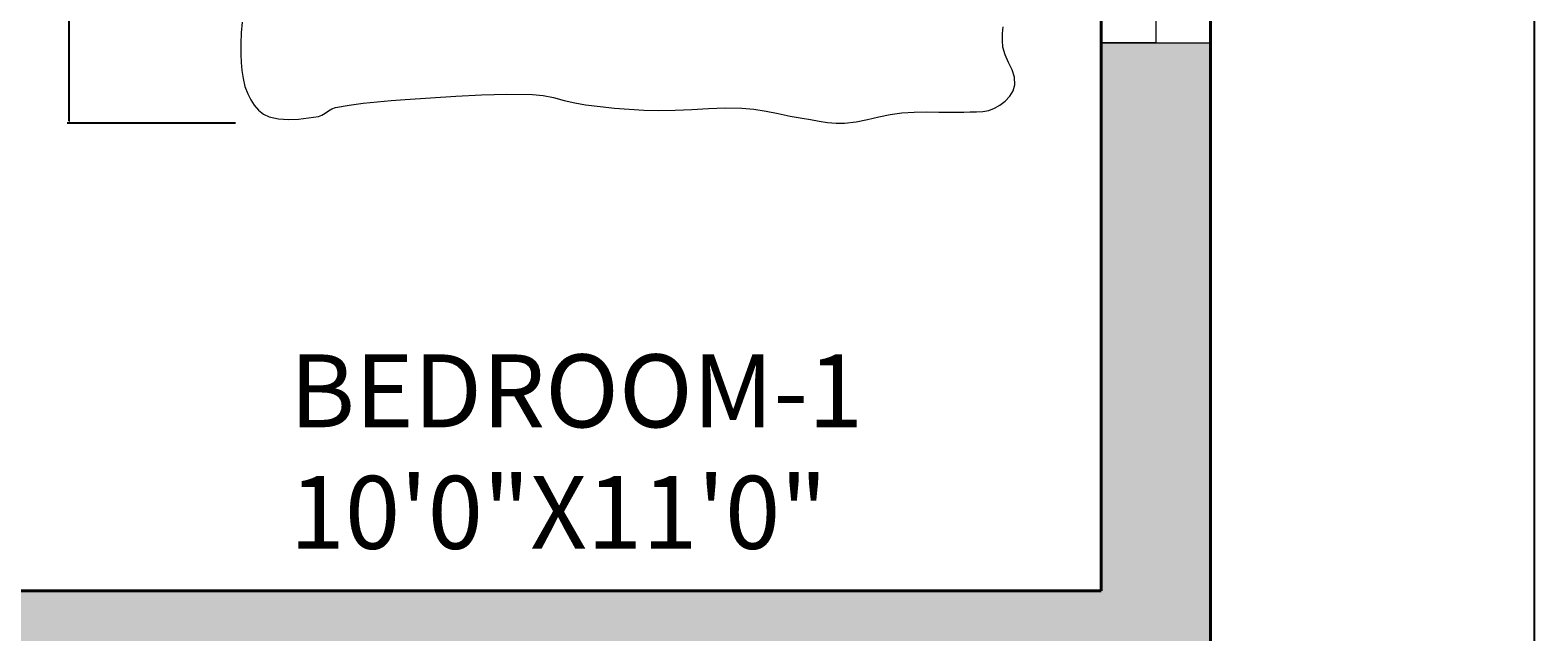
# Model space of a CAD drawing. Units: inches. Extents: x 1441 to 2460, y 1648 to 2683.
# Tile 22 of 35: x 1792 to 1916, y 2154 to 2204. Entities that reach past the tile are written whole.
import ezdxf

# ---------------------------------------------------------------- set-up
doc = ezdxf.new("R2010")
doc.units = ezdxf.units.IN
for name, color, linetype, lineweight in [('A-ANNO-DIMS', 2, 'Continuous', 18), ('A-AREA-IDEN', 7, 'Continuous', 20), ('A-FURN', 8, 'Continuous', 15), ('A-GLAZ', 4, 'Continuous', 18), ('A-WALL', 7, 'Continuous', 40)]:
    doc.layers.add(name, color=color, linetype=linetype, lineweight=lineweight)
doc.layers.add('A-WALL-PATT', color=251, linetype='Continuous', lineweight=13, true_color=0x636466)
doc.styles.get("Standard").update_dxf_attribs({"font": 'arial.ttf'})
doc.dimstyles.get("Standard").update_dxf_attribs({"dimtxt": 0.18, "dimasz": 0.18, "dimexe": 0.18, "dimexo": 0.0625, "dimgap": 0.09, "dimtad": 0, "dimtih": 1, "dimtoh": 1, "dimdec": 4, "dimzin": 0, "dimdsep": 46, "dimtxsty": 'Standard', "dimcen": 0.09, "dimadec": 0, "dimazin": 0, "dimtfac": 1, "dimtdec": 4, "dimtofl": 0, "dimtmove": 0, "dimatfit": 3, "dimfxl": 1, "dimtolj": 1, "dimtzin": 0, "dimarcsym": 0})

# ---------------------------------------------------------------- blocks, each defined once
blk = doc.blocks.new('BED-DOUBLE-PLAN')
for p, q in [((0.48, 8.33), (0.41, 7.44)), ((63.07, 7.38), (63.12, 7.94)), ((0.41, 7.44), (0.36, 6.56)), ((0.36, 6.56), (0.37, 5.67)), ((63.06, 6.82), (63.07, 7.38)), ((63.1, 6.26), (63.06, 6.82)), ((63.28, 5.62), (63.1, 6.26)), ((0.37, 5.67), (0.4, 5)), ((0.4, 5), (0.46, 4.34)), ((63.56, 5.01), (63.28, 5.62)), ((63.86, 4.4), (63.56, 5.01)), ((0.46, 4.34), (0.56, 3.68)), ((64.07, 3.78), (63.86, 4.4)), ((64.1, 3.15), (64.07, 3.78)), ((0.56, 3.68), (0.71, 3.03)), ((0.71, 3.03), (0.94, 2.41)), ((63.67, 2.22), (63.96, 2.66)), ((63.96, 2.66), (64.1, 3.15)), ((0.94, 2.41), (1.18, 1.94)), ((1.18, 1.94), (1.48, 1.49)), ((1.48, 1.49), (1.83, 1.09)), ((7.85, 1.2), (8.15, 1.31)), ((8.15, 1.31), (9.29, 1.5)), ((9.29, 1.5), (10.43, 1.66)), ((10.43, 1.66), (11.58, 1.77)), ((11.58, 1.77), (12.74, 1.87)), ((12.74, 1.87), (13.89, 1.95)), ((13.89, 1.95), (15.99, 2.09)), ((15.99, 2.09), (18.08, 2.23)), ((18.08, 2.23), (20.17, 2.34)), ((20.17, 2.34), (22.27, 2.4)), ((22.27, 2.4), (24.37, 2.38)), ((24.37, 2.38), (25.25, 2.29)), ((25.25, 2.29), (26.12, 2.11)), ((26.12, 2.11), (26.99, 1.88)), ((26.99, 1.88), (27.86, 1.67)), ((27.86, 1.67), (28.74, 1.51)), ((28.74, 1.51), (29.94, 1.37)), ((29.94, 1.37), (31.14, 1.25)), ((31.14, 1.25), (32.35, 1.16)), ((38.87, 1.22), (40.25, 1.28)), ((40.25, 1.28), (41.62, 1.25)), ((41.62, 1.25), (42.61, 1.16)), ((62.41, 1.23), (62.86, 1.5)), ((62.86, 1.5), (63.3, 1.83)), ((63.3, 1.83), (63.67, 2.22)), ((1.83, 1.09), (2.23, 0.76)), ((2.23, 0.76), (2.69, 0.54)), ((2.69, 0.54), (3.48, 0.36)), ((3.48, 0.36), (4.29, 0.31)), ((4.29, 0.31), (5.11, 0.35)), ((5.11, 0.35), (5.93, 0.45)), ((5.93, 0.45), (6.75, 0.56)), ((6.75, 0.56), (7.04, 0.66)), ((7.04, 0.66), (7.32, 0.83)), ((7.32, 0.83), (7.58, 1.03)), ((7.58, 1.03), (7.85, 1.2)), ((32.35, 1.16), (33.55, 1.09)), ((33.55, 1.09), (34.76, 1.05)), ((34.76, 1.05), (36.13, 1.07)), ((36.13, 1.07), (37.5, 1.14)), ((37.5, 1.14), (38.87, 1.22)), ((42.61, 1.16), (43.61, 0.99)), ((43.61, 0.99), (44.6, 0.79)), ((44.6, 0.79), (45.58, 0.59)), ((45.58, 0.59), (46.58, 0.41)), ((46.58, 0.41), (47.27, 0.3)), ((47.27, 0.3), (47.97, 0.18)), ((47.97, 0.18), (48.67, 0.07)), ((48.67, 0.07), (49.37, 0)), ((49.37, 0), (50.07, 0)), ((50.07, 0), (51.02, 0.11)), ((51.02, 0.11), (51.96, 0.3)), ((51.96, 0.3), (52.89, 0.52)), ((52.89, 0.52), (53.83, 0.73)), ((53.83, 0.73), (54.78, 0.86)), ((54.78, 0.86), (55.8, 0.92)), ((55.8, 0.92), (56.82, 0.93)), ((56.82, 0.93), (57.84, 0.91)), ((57.84, 0.91), (58.87, 0.9)), ((58.87, 0.9), (59.89, 0.92)), ((59.89, 0.92), (60.41, 0.93)), ((60.41, 0.93), (60.93, 0.93)), ((60.93, 0.93), (61.44, 0.96)), ((61.44, 0.96), (61.94, 1.05)), ((61.94, 1.05), (62.41, 1.23))]:
    blk.add_line(p, q)
blk = doc.blocks.new('WIN-48-SASH')
for p, q in [((9, 48), (4.5, 48)), ((4.5, 48), (4.5, 0)), ((4.5, 0), (0, 0))]:
    blk.add_line(p, q)
blk = doc.blocks.new('*D22')
at = {"layer": 'A-ANNO-DIMS', "color": 0, "lineweight": -2, "transparency": 16777216}
for p, q in [((1809.14, 2287.87), (1795.27, 2287.87)), ((1795.45, 2287.69), (1795.45, 2242.21)), ((1795.45, 2196.36), (1795.45, 2241.84)), ((1809.14, 2196.18), (1795.27, 2196.18))]:
    blk.add_line(p, q, dxfattribs=at)
at = {"layer": 'A-ANNO-DIMS', "color": 0, "transparency": 16777216}
for points in [[(1795.42, 2287.69), (1795.48, 2287.69), (1795.45, 2287.87)], [(1795.42, 2196.36), (1795.48, 2196.36), (1795.45, 2196.18)]]:
    blk.add_solid(points, dxfattribs=at)
at = {"layer": 'Defpoints', "color": 0, "transparency": 16777216}
for p in [(1795.45, 2287.87), (1809.2, 2287.87), (1809.2, 2196.18)]:
    blk.add_point(p, dxfattribs=at)
at = {"layer": 'A-ANNO-DIMS', "color": 0, "transparency": 16777216, "insert": (1795.45, 2242.03), "char_height": 0.18, "attachment_point": 5}
blk.add_mtext('\\A1;DOUBLE BED 92 TYP.', dxfattribs=at)
blk = doc.blocks.new('*D67')
at = {"layer": 'A-ANNO-DIMS', "color": 0, "lineweight": -2, "transparency": 16777216}
for p, q in [((1889.45, 2298.7), (1916.22, 2298.7)), ((1916.04, 2298.52), (1916.04, 2055.94)), ((1916.04, 1813), (1916.04, 2055.57)), ((1758.22, 1812.82), (1916.22, 1812.82))]:
    blk.add_line(p, q, dxfattribs=at)
at = {"layer": 'A-ANNO-DIMS', "color": 0, "transparency": 16777216}
for points in [[(1916.01, 2298.52), (1916.07, 2298.52), (1916.04, 2298.7)], [(1916.01, 1813), (1916.07, 1813), (1916.04, 1812.82)]]:
    blk.add_solid(points, dxfattribs=at)
at = {"layer": 'Defpoints', "color": 0, "transparency": 16777216}
for p in [(1889.39, 2298.7), (1916.04, 2298.7), (1758.16, 1812.82)]:
    blk.add_point(p, dxfattribs=at)
at = {"layer": 'A-ANNO-DIMS', "color": 0, "transparency": 16777216, "insert": (1916.04, 2055.76), "char_height": 0.18, "attachment_point": 5}
blk.add_mtext('\\A1;485.9', dxfattribs=at)

msp = doc.modelspace()

# ---------------------------------------------------------------- hatches: boundary and pattern name
at = {"layer": 'A-WALL-PATT'}
h = msp.add_hatch(color=256, dxfattribs=at)
h.dxf.hatch_style = 1
h.paths.add_polyline_path([(1627.5085, 2298.6952), (1568.8859, 2298.6952), (1568.8859, 2246.9605), (1577.8859, 2246.9605), (1577.8859, 2289.6952), (1627.5085, 2289.6952), (1627.5085, 2294.1952)])
h.paths.add_polyline_path([(1675.5777, 2298.6952), (1651.5085, 2298.6952), (1651.5085, 2289.6952), (1675.5777, 2289.6952), (1675.5777, 2294.1952)])
h.paths.add_polyline_path([(1667.3859, 2289.6952), (1662.8859, 2289.6952), (1662.8859, 2233.0622), (1667.3859, 2233.0622)])
h.paths.add_polyline_path([(1715.8721, 2294.3362), (1715.8721, 2295.2788), (1715.8721, 2298.6952), (1699.5777, 2298.6952), (1699.5777, 2289.6952), (1715.8721, 2289.6952)])
h.paths.add_polyline_path([(1707.8859, 2289.6952), (1703.3859, 2289.6952), (1703.3859, 2199.6952), (1707.8859, 2199.6952)])
h.paths.add_polyline_path([(1760.3859, 2204.637), (1755.8859, 2204.637), (1755.8859, 2199.6952), (1667.3859, 2199.6952), (1667.3859, 2204.637), (1662.8859, 2204.637), (1662.8859, 2195.1952), (1760.3859, 2195.1952)])
h.paths.add_polyline_path([(1760.3859, 2289.6952), (1755.8859, 2289.6952), (1755.8859, 2233.0622), (1760.3859, 2233.0622)])
h.paths.add_polyline_path([(1889.3859, 2298.6952), (1739.8721, 2298.6952), (1739.8721, 2289.6952), (1880.3859, 2289.6952), (1880.3859, 2250.8051), (1889.3859, 2250.8051)])
h.paths.add_polyline_path([(1889.3859, 2202.8051), (1880.3859, 2202.8051), (1880.3859, 2157.6952), (1747.948, 2157.6952), (1747.948, 2153.1952), (1755.8859, 2153.1952), (1755.8859, 2058.005), (1760.3859, 2058.005), (1760.3859, 2153.1952), (1880.3859, 2153.1952), (1880.3859, 2124.108), (1889.3859, 2124.108)])
h.paths.add_polyline_path([(1889.3859, 1984.8305), (1880.3859, 1984.8305), (1880.3859, 1834.1952), (1889.3859, 1834.1952)])
h.paths.add_polyline_path([(1889.3859, 2076.108), (1880.3859, 2076.108), (1880.3859, 2008.8305), (1889.3859, 2008.8305)])
h.paths.add_polyline_path([(1880.3859, 2027.1952), (1800.8859, 2027.1952), (1800.8859, 2000.9452), (1805.3859, 2000.9452), (1805.3859, 2022.6952), (1880.3859, 2022.6952)])
h.paths.add_polyline_path([(1800.8859, 2027.1952), (1760.3859, 2027.1952), (1760.3859, 2030.7912), (1755.8859, 2030.7912), (1755.8859, 2022.6952), (1800.8859, 2022.6952)])
h.paths.add_polyline_path([(1880.3859, 1974.6952), (1805.3859, 1974.6952), (1805.3859, 1978.7973), (1800.8859, 1978.7973), (1800.8859, 1974.6952), (1794.8823, 1974.6952), (1794.8823, 1970.1952), (1800.8859, 1970.1952), (1805.3859, 1970.1952), (1880.3859, 1970.1952)])
h.paths.add_polyline_path([(1760.3859, 1974.6952), (1755.8859, 1974.6952), (1755.8859, 1925.6952), (1751.8616, 1925.6952), (1751.8616, 1921.1952), (1760.3859, 1921.1952)])
h.paths.add_polyline_path([(1760.3859, 1921.1952), (1755.8859, 1921.1952), (1755.8859, 1843.1952), (1760.3859, 1843.1952)])
h.paths.add_polyline_path([(1799.1136, 1838.6952), (1799.1136, 1843.1952), (1760.3859, 1843.1952), (1751.8944, 1843.1952), (1751.8944, 1834.1952), (1758.1615, 1834.1952), (1799.1136, 1834.1952)])
h.paths.add_polyline_path([(1880.3859, 1843.1952), (1859.1136, 1843.1952), (1859.1136, 1834.1952), (1880.3859, 1834.1952)])
h.paths.add_polyline_path([(1577.8859, 1857.7914), (1568.8859, 1857.7914), (1568.8859, 1834.1952), (1695.0034, 1834.1952), (1695.0034, 1838.6952), (1695.0034, 1843.1952), (1577.8859, 1843.1952)])
h.paths.add_polyline_path([(1577.8859, 1959.2399), (1573.3859, 1959.2399), (1568.8859, 1959.2399), (1568.8859, 1905.7914), (1577.8859, 1905.7914), (1577.8859, 1921.1952), (1703.3859, 1921.1952), (1707.8859, 1921.1952), (1715.1501, 1921.1952), (1715.1501, 1925.6952), (1707.8859, 1925.6952), (1703.3859, 1925.6952), (1577.8859, 1925.6952)])
h.paths.add_polyline_path([(1577.8859, 2106.6907), (1568.8859, 2106.6907), (1568.8859, 2019.2399), (1577.8859, 2019.2399)])
h.paths.add_polyline_path([(1707.8859, 2051.6952), (1703.3859, 2051.6952), (1703.3859, 2048.6952), (1703.3859, 1925.6952), (1707.8859, 1925.6952)])
h.paths.add_polyline_path([(1703.3859, 2051.6952), (1676.3859, 2051.6952), (1676.3859, 2048.6952), (1703.3859, 2048.6952)])
h.paths.add_polyline_path([(1703.3859, 2102.6952), (1676.3859, 2102.6952), (1676.3859, 2099.6952), (1685.3859, 2099.6952), (1703.3859, 2099.6952)])
h.paths.add_polyline_path([(1707.8859, 2153.1952), (1710.5611, 2153.1952), (1710.5611, 2157.6952), (1707.8859, 2157.6952), (1707.8859, 2195.1952), (1703.3859, 2195.1952), (1703.3859, 2099.6952), (1707.8859, 2099.6952)])
h.paths.add_polyline_path([(1577.8859, 2198.9605), (1568.8859, 2198.9605), (1568.8859, 2166.6907), (1577.8859, 2166.6907)])

# ---------------------------------------------------------------- linework, layer by layer
at = {"layer": 'A-GLAZ'}
msp.add_line((1880.3859, 2202.8051), (1889.3859, 2202.8051), dxfattribs=at)
at = {"layer": 'A-WALL'}
for p, q in [((1889.3859, 2298.6952), (1889.3859, 1834.1952)), ((1880.3859, 2289.6952), (1880.3859, 2157.6952)), ((1880.3859, 2195.1952), (1880.3859, 2157.6952)), ((1747.948, 2157.6952), (1880.3859, 2157.6952))]:
    msp.add_line(p, q, dxfattribs=at)

# ---------------------------------------------------------------- block references
at = {"layer": 'A-FURN'}
msp.add_blockref('BED-DOUBLE-PLAN', (1809.2, 2196.18), dxfattribs=at)
at = {"layer": 'A-GLAZ'}
msp.add_blockref('WIN-48-SASH', (1880.39, 2202.8045), dxfattribs=at)

# ---------------------------------------------------------------- texts
at = {"layer": 'A-AREA-IDEN', "insert": (1813.5956, 2177.1552), "char_height": 6, "attachment_point": 1}
msp.add_mtext_dynamic_manual_height_columns('BEDROOM-1\\P10\'0"X11\'0"', width=85.554017, gutter_width=12.5, heights=[0], dxfattribs=at)

# ---------------------------------------------------------------- dimensions: what is measured, and where the dimension line sits
at = {"layer": 'A-ANNO-DIMS'}
dim = msp.add_linear_dim(base=(1916.0359, 2298.6952), p1=(1758.1615, 1812.8171), p2=(1889.3859, 2298.6952), angle=90, dimstyle='Standard', override={"dimdec": 1, "dimlfac": 1, "dimrnd": 0, "dimzin": 0, "dimdsep": 46, "dimlunit": 2}, dxfattribs=at)
dim.commit()
dim.dimension.update_dxf_attribs({"geometry": '*D67', "text_midpoint": (1916.0359, 2055.7561)})
dim = msp.add_linear_dim(base=(1795.4489, 2287.8701), p1=(1809.2021, 2196.1822), p2=(1809.2021, 2287.8701), angle=90, text='DOUBLE BED <> TYP.', dimstyle='Standard', override={"dimdec": 0, "dimlfac": 1, "dimrnd": 0, "dimzin": 0, "dimdsep": 46, "dimlunit": 2}, dxfattribs=at)
dim.commit()
dim.dimension.update_dxf_attribs({"geometry": '*D22', "text_midpoint": (1795.4489, 2242.0262)})

doc.saveas('drawing.dxf')
